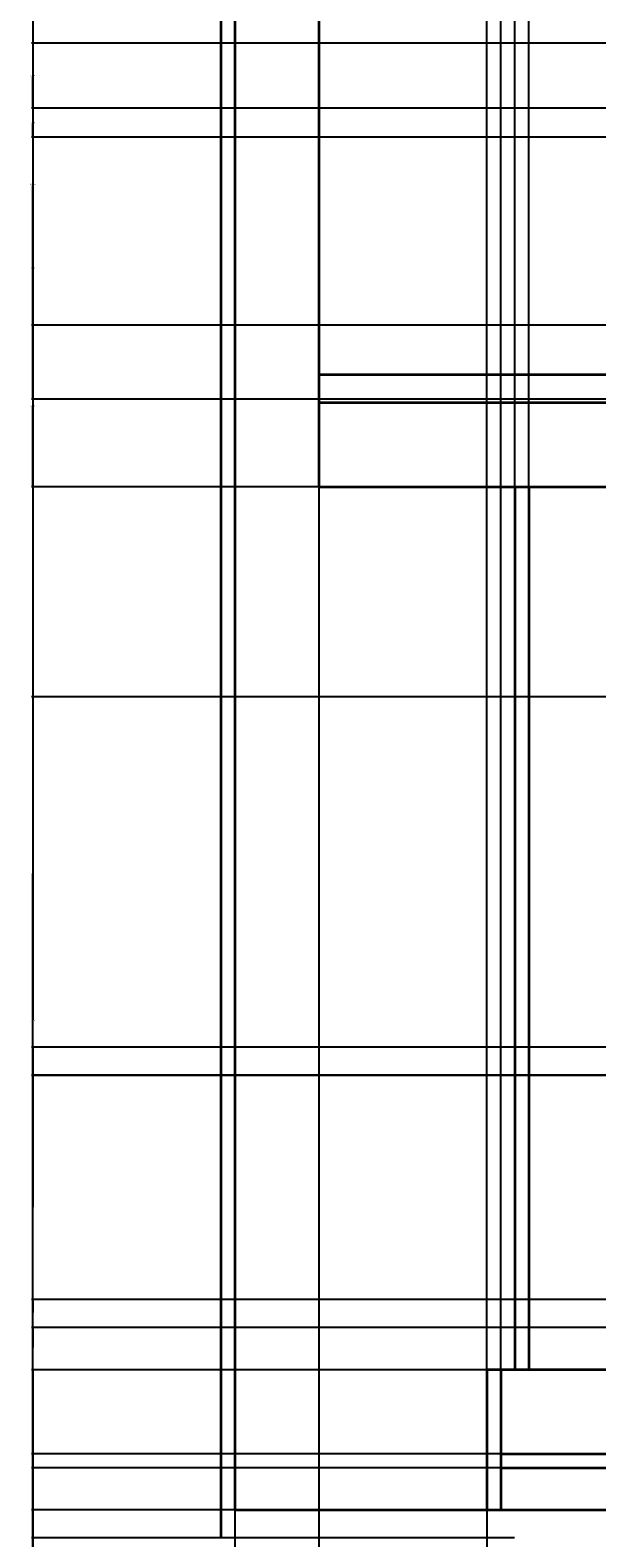
# Model space of a CAD drawing. Units: inches. Extents: x 2154 to 2740, y 571 to 1084.
# Tile 2 of 13: x 2154 to 2235, y 754 to 969. Entities that reach past the tile are written whole.
import ezdxf

# ---------------------------------------------------------------- set-up
doc = ezdxf.new("R2010")
doc.units = ezdxf.units.IN
for name, color, linetype, lineweight in [('A-ANNO-DIMS', 2, 'Continuous', 18), ('A-ELEV', 7, 'Continuous', 35), ('A-ROOF', 1, 'Continuous', 35)]:
    doc.layers.add(name, color=color, linetype=linetype, lineweight=lineweight)
doc.styles.get("Standard").update_dxf_attribs({"font": 'arial.ttf'})
doc.dimstyles.get("Standard").update_dxf_attribs({"dimtxt": 0.18, "dimasz": 0.18, "dimexe": 0.18, "dimexo": 0.0625, "dimgap": 0.09, "dimtad": 0, "dimtih": 1, "dimtoh": 1, "dimdec": 4, "dimzin": 0, "dimdsep": 46, "dimtxsty": 'Standard', "dimcen": 0.09, "dimadec": 0, "dimazin": 0, "dimtfac": 1, "dimtdec": 4, "dimtofl": 0, "dimtmove": 0, "dimatfit": 3, "dimfxl": 1, "dimtolj": 1, "dimtzin": 0, "dimarcsym": 0})

# ---------------------------------------------------------------- blocks, each defined once
blk = doc.blocks.new('*D10')
at = {"layer": 'A-ANNO-DIMS', "color": 0, "lineweight": -2, "transparency": 16777216}
for p, q in [((2447.14, 1057.01), (2154.18, 1057.01)), ((2154.36, 1056.83), (2154.36, 827.45)), ((2154.36, 597.71), (2154.36, 827.09)), ((2181.14, 597.53), (2154.18, 597.53))]:
    blk.add_line(p, q, dxfattribs=at)
at = {"layer": 'A-ANNO-DIMS', "color": 0, "transparency": 16777216}
for points in [[(2154.33, 1056.83), (2154.39, 1056.83), (2154.36, 1057.01)], [(2154.33, 597.71), (2154.39, 597.71), (2154.36, 597.53)]]:
    blk.add_solid(points, dxfattribs=at)
at = {"layer": 'Defpoints', "color": 0, "transparency": 16777216}
for p in [(2154.36, 1057.01), (2447.21, 1057.01), (2181.21, 597.53)]:
    blk.add_point(p, dxfattribs=at)
at = {"layer": 'A-ANNO-DIMS', "color": 0, "transparency": 16777216, "insert": (2154.36, 827.27), "char_height": 0.18, "attachment_point": 5}
blk.add_mtext('\\A1;459.5', dxfattribs=at)
blk = doc.blocks.new('*D14')
at = {"layer": 'A-ANNO-DIMS', "color": 0, "lineweight": -2, "transparency": 16777216}
for p, q in [((2221.14, 777.53), (2154.18, 777.53)), ((2154.36, 777.35), (2154.36, 687.71)), ((2154.36, 597.71), (2154.36, 687.35)), ((2223.14, 597.53), (2154.18, 597.53))]:
    blk.add_line(p, q, dxfattribs=at)
at = {"layer": 'A-ANNO-DIMS', "color": 0, "transparency": 16777216}
for points in [[(2154.33, 777.35), (2154.39, 777.35), (2154.36, 777.53)], [(2154.33, 597.71), (2154.39, 597.71), (2154.36, 597.53)]]:
    blk.add_solid(points, dxfattribs=at)
at = {"layer": 'Defpoints', "color": 0, "transparency": 16777216}
for p in [(2154.36, 777.53), (2221.21, 777.53), (2223.21, 597.53)]:
    blk.add_point(p, dxfattribs=at)
at = {"layer": 'A-ANNO-DIMS', "color": 0, "transparency": 16777216, "insert": (2154.36, 687.53), "char_height": 0.18, "attachment_point": 5}
blk.add_mtext('\\A1;180', dxfattribs=at)
blk = doc.blocks.new('*D15')
at = {"layer": 'A-ANNO-DIMS', "color": 0, "lineweight": -2, "transparency": 16777216}
for p, q in [((2223.14, 903.53), (2154.18, 903.53)), ((2154.36, 903.35), (2154.36, 840.71)), ((2154.36, 777.71), (2154.36, 840.35)), ((2221.14, 777.53), (2154.18, 777.53))]:
    blk.add_line(p, q, dxfattribs=at)
at = {"layer": 'A-ANNO-DIMS', "color": 0, "transparency": 16777216}
for points in [[(2154.33, 903.35), (2154.39, 903.35), (2154.36, 903.53)], [(2154.33, 777.71), (2154.39, 777.71), (2154.36, 777.53)]]:
    blk.add_solid(points, dxfattribs=at)
at = {"layer": 'Defpoints', "color": 0, "transparency": 16777216}
for p in [(2154.36, 903.53), (2223.21, 903.53), (2221.21, 777.53)]:
    blk.add_point(p, dxfattribs=at)
at = {"layer": 'A-ANNO-DIMS', "color": 0, "transparency": 16777216, "insert": (2154.36, 840.53), "char_height": 0.18, "attachment_point": 5}
blk.add_mtext('\\A1;126', dxfattribs=at)
blk = doc.blocks.new('*D30')
at = {"layer": 'A-ANNO-DIMS', "color": 0, "lineweight": -2, "transparency": 16777216}
for p, q in [((2657.14, 823.53), (2154.18, 823.53)), ((2154.36, 823.35), (2154.36, 800.71)), ((2154.36, 777.71), (2154.36, 800.35)), ((2657.14, 777.53), (2154.18, 777.53))]:
    blk.add_line(p, q, dxfattribs=at)
at = {"layer": 'A-ANNO-DIMS', "color": 0, "transparency": 16777216}
for points in [[(2154.33, 823.35), (2154.39, 823.35), (2154.36, 823.53)], [(2154.33, 777.71), (2154.39, 777.71), (2154.36, 777.53)]]:
    blk.add_solid(points, dxfattribs=at)
at = {"layer": 'Defpoints', "color": 0, "transparency": 16777216}
for p in [(2154.36, 823.53), (2657.21, 823.53), (2657.21, 777.53)]:
    blk.add_point(p, dxfattribs=at)
at = {"layer": 'A-ANNO-DIMS', "color": 0, "transparency": 16777216, "insert": (2154.36, 800.53), "char_height": 0.18, "attachment_point": 5}
blk.add_mtext('\\A1;46', dxfattribs=at)
blk = doc.blocks.new('*D33')
at = {"layer": 'A-ANNO-DIMS', "color": 0, "lineweight": -2, "transparency": 16777216}
for p, q in [((2412.64, 873.53), (2154.18, 873.53)), ((2154.36, 873.35), (2154.36, 848.71)), ((2154.36, 823.71), (2154.36, 848.35)), ((2412.64, 823.53), (2154.18, 823.53))]:
    blk.add_line(p, q, dxfattribs=at)
at = {"layer": 'A-ANNO-DIMS', "color": 0, "transparency": 16777216}
for points in [[(2154.33, 873.35), (2154.39, 873.35), (2154.36, 873.53)], [(2154.33, 823.71), (2154.39, 823.71), (2154.36, 823.53)]]:
    blk.add_solid(points, dxfattribs=at)
at = {"layer": 'Defpoints', "color": 0, "transparency": 16777216}
for p in [(2154.36, 873.53), (2412.71, 873.53), (2412.71, 823.53)]:
    blk.add_point(p, dxfattribs=at)
at = {"layer": 'A-ANNO-DIMS', "color": 0, "transparency": 16777216, "insert": (2154.36, 848.53), "char_height": 0.18, "attachment_point": 5}
blk.add_mtext('\\A1;50', dxfattribs=at)
blk = doc.blocks.new('*D35')
at = {"layer": 'A-ANNO-DIMS', "color": 0, "lineweight": -2, "transparency": 16777216}
for p, q in [((2447.21, 966.82), (2154.18, 966.82)), ((2154.36, 966.64), (2154.36, 946.87)), ((2154.36, 926.74), (2154.36, 946.51)), ((2284.14, 926.56), (2154.18, 926.56))]:
    blk.add_line(p, q, dxfattribs=at)
at = {"layer": 'A-ANNO-DIMS', "color": 0, "transparency": 16777216}
for points in [[(2154.33, 966.64), (2154.39, 966.64), (2154.36, 966.82)], [(2154.33, 926.74), (2154.39, 926.74), (2154.36, 926.56)]]:
    blk.add_solid(points, dxfattribs=at)
at = {"layer": 'Defpoints', "color": 0, "transparency": 16777216}
for p in [(2154.36, 966.82), (2447.27, 966.82), (2284.21, 926.56)]:
    blk.add_point(p, dxfattribs=at)
at = {"layer": 'A-ANNO-DIMS', "color": 0, "transparency": 16777216, "insert": (2154.36, 946.69), "char_height": 0.18, "attachment_point": 5}
blk.add_mtext('\\A1;40.255', dxfattribs=at)
blk = doc.blocks.new('*D36')
at = {"layer": 'A-ANNO-DIMS', "color": 0, "lineweight": -2, "transparency": 16777216}
for p, q in [((2447.21, 966.82), (2154.18, 966.82)), ((2154.36, 966.64), (2154.36, 962.36)), ((2154.36, 957.71), (2154.36, 961.99)), ((2447.14, 957.53), (2154.18, 957.53))]:
    blk.add_line(p, q, dxfattribs=at)
at = {"layer": 'A-ANNO-DIMS', "color": 0, "transparency": 16777216}
for points in [[(2154.33, 966.64), (2154.39, 966.64), (2154.36, 966.82)], [(2154.33, 957.71), (2154.39, 957.71), (2154.36, 957.53)]]:
    blk.add_solid(points, dxfattribs=at)
at = {"layer": 'Defpoints', "color": 0, "transparency": 16777216}
for p in [(2154.36, 966.82), (2447.27, 966.82), (2447.21, 957.53)]:
    blk.add_point(p, dxfattribs=at)
at = {"layer": 'A-ANNO-DIMS', "color": 0, "transparency": 16777216, "insert": (2154.36, 962.18), "char_height": 0.18, "attachment_point": 5}
blk.add_mtext('\\A1;9.287', dxfattribs=at)
blk = doc.blocks.new('*D37')
at = {"layer": 'A-ANNO-DIMS', "color": 0, "lineweight": -2, "transparency": 16777216}
for p, q in [((2447.14, 957.53), (2154.18, 957.53)), ((2154.36, 957.35), (2154.36, 955.65)), ((2154.36, 953.58), (2154.36, 955.29)), ((2447.11, 953.4), (2154.18, 953.4))]:
    blk.add_line(p, q, dxfattribs=at)
at = {"layer": 'A-ANNO-DIMS', "color": 0, "transparency": 16777216}
for points in [[(2154.33, 957.35), (2154.39, 957.35), (2154.36, 957.53)], [(2154.33, 953.58), (2154.39, 953.58), (2154.36, 953.4)]]:
    blk.add_solid(points, dxfattribs=at)
at = {"layer": 'Defpoints', "color": 0, "transparency": 16777216}
for p in [(2154.36, 957.53), (2447.21, 957.53), (2447.18, 953.4)]:
    blk.add_point(p, dxfattribs=at)
at = {"layer": 'A-ANNO-DIMS', "color": 0, "transparency": 16777216, "insert": (2154.36, 955.47), "char_height": 0.18, "attachment_point": 5}
blk.add_mtext('\\A1;4.127', dxfattribs=at)
blk = doc.blocks.new('*D38')
at = {"layer": 'A-ANNO-DIMS', "color": 0, "lineweight": -2, "transparency": 16777216}
for p, q in [((2447.11, 953.4), (2154.18, 953.4)), ((2154.36, 953.22), (2154.36, 934.9)), ((2154.36, 916.21), (2154.36, 934.53)), ((2295.71, 916.03), (2154.18, 916.03))]:
    blk.add_line(p, q, dxfattribs=at)
at = {"layer": 'A-ANNO-DIMS', "color": 0, "transparency": 16777216}
for points in [[(2154.33, 953.22), (2154.39, 953.22), (2154.36, 953.4)], [(2154.33, 916.21), (2154.39, 916.21), (2154.36, 916.03)]]:
    blk.add_solid(points, dxfattribs=at)
at = {"layer": 'Defpoints', "color": 0, "transparency": 16777216}
for p in [(2154.36, 953.4), (2447.18, 953.4), (2295.77, 916.03)]:
    blk.add_point(p, dxfattribs=at)
at = {"layer": 'A-ANNO-DIMS', "color": 0, "transparency": 16777216, "insert": (2154.36, 934.72), "char_height": 0.18, "attachment_point": 5}
blk.add_mtext('\\A1;37.38', dxfattribs=at)
blk = doc.blocks.new('*D39')
at = {"layer": 'A-ANNO-DIMS', "color": 0, "lineweight": -2, "transparency": 16777216}
for p, q in [((2183.21, 979.47), (2183.21, 570.5)), ((2417.21, 970.47), (2417.21, 570.5)), ((2183.39, 570.68), (2299.92, 570.68)), ((2417.03, 570.68), (2300.5, 570.68))]:
    blk.add_line(p, q, dxfattribs=at)
at = {"layer": 'A-ANNO-DIMS', "color": 0, "transparency": 16777216}
for points in [[(2183.39, 570.71), (2183.39, 570.65), (2183.21, 570.68)], [(2417.03, 570.71), (2417.03, 570.65), (2417.21, 570.68)]]:
    blk.add_solid(points, dxfattribs=at)
at = {"layer": 'Defpoints', "color": 0, "transparency": 16777216}
for p in [(2183.21, 979.53), (2417.21, 970.53), (2417.21, 570.68)]:
    blk.add_point(p, dxfattribs=at)
at = {"layer": 'A-ANNO-DIMS', "color": 0, "transparency": 16777216, "insert": (2300.21, 570.68), "char_height": 0.18, "attachment_point": 5}
blk.add_mtext('\\A1;234', dxfattribs=at)
blk = doc.blocks.new('*D46')
at = {"layer": 'A-ANNO-DIMS', "color": 0, "lineweight": -2, "transparency": 16777216}
for p, q in [((2195.27, 915.53), (2740.24, 915.53)), ((2740.06, 915.35), (2740.06, 909.71)), ((2740.06, 903.71), (2740.06, 909.35)), ((2195.27, 903.53), (2740.24, 903.53))]:
    blk.add_line(p, q, dxfattribs=at)
at = {"layer": 'A-ANNO-DIMS', "color": 0, "transparency": 16777216}
for points in [[(2740.03, 915.35), (2740.09, 915.35), (2740.06, 915.53)], [(2740.03, 903.71), (2740.09, 903.71), (2740.06, 903.53)]]:
    blk.add_solid(points, dxfattribs=at)
at = {"layer": 'Defpoints', "color": 0, "transparency": 16777216}
for p in [(2195.21, 915.53), (2740.06, 915.53), (2195.21, 903.53)]:
    blk.add_point(p, dxfattribs=at)
at = {"layer": 'A-ANNO-DIMS', "color": 0, "transparency": 16777216, "insert": (2740.06, 909.53), "char_height": 0.18, "attachment_point": 5}
blk.add_mtext('\\A1;12', dxfattribs=at)
blk = doc.blocks.new('*D47')
at = {"layer": 'A-ANNO-DIMS', "color": 0, "lineweight": -2, "transparency": 16777216}
for p, q in [((2195.269199, 919.532069), (2740.236699, 919.532069)), ((2740.056699, 919.352069), (2740.056699, 917.712069)), ((2740.056699, 915.712069), (2740.056699, 917.352069)), ((2195.269199, 915.532069), (2740.236699, 915.532069))]:
    blk.add_line(p, q, dxfattribs=at)
at = {"layer": 'A-ANNO-DIMS', "color": 0, "transparency": 16777216}
for points in [[(2740.026699, 919.352069), (2740.086699, 919.352069), (2740.056699, 919.532069)], [(2740.026699, 915.712069), (2740.086699, 915.712069), (2740.056699, 915.532069)]]:
    blk.add_solid(points, dxfattribs=at)
at = {"layer": 'Defpoints', "color": 0, "transparency": 16777216}
for p in [(2195.206699, 919.532069), (2740.056699, 919.532069), (2195.206699, 915.532069)]:
    blk.add_point(p, dxfattribs=at)
at = {"layer": 'A-ANNO-DIMS', "color": 0, "transparency": 16777216, "insert": (2740.056699, 917.532069), "char_height": 0.18, "attachment_point": 5}
blk.add_mtext('\\A1;4', dxfattribs=at)
blk = doc.blocks.new('*D48')
at = {"layer": 'A-ANNO-DIMS', "color": 0, "lineweight": -2, "transparency": 16777216}
for p, q in [((2195.27, 979.53), (2740.24, 979.53)), ((2740.06, 979.35), (2740.06, 949.71)), ((2740.06, 919.71), (2740.06, 949.35)), ((2195.27, 919.53), (2740.24, 919.53))]:
    blk.add_line(p, q, dxfattribs=at)
at = {"layer": 'A-ANNO-DIMS', "color": 0, "transparency": 16777216}
for points in [[(2740.03, 979.35), (2740.09, 979.35), (2740.06, 979.53)], [(2740.03, 919.71), (2740.09, 919.71), (2740.06, 919.53)]]:
    blk.add_solid(points, dxfattribs=at)
at = {"layer": 'Defpoints', "color": 0, "transparency": 16777216}
for p in [(2195.21, 979.53), (2740.06, 979.53), (2195.21, 919.53)]:
    blk.add_point(p, dxfattribs=at)
at = {"layer": 'A-ANNO-DIMS', "color": 0, "transparency": 16777216, "insert": (2740.06, 949.53), "char_height": 0.18, "attachment_point": 5}
blk.add_mtext('\\A1;60', dxfattribs=at)
blk = doc.blocks.new('*D51')
at = {"layer": 'A-ANNO-DIMS', "color": 0, "lineweight": -2, "transparency": 16777216}
for p, q in [((2183.21, 979.47), (2183.21, 570.5)), ((2195.21, 979.47), (2195.21, 570.5)), ((2183.39, 570.68), (2189, 570.68)), ((2195.03, 570.68), (2189.42, 570.68))]:
    blk.add_line(p, q, dxfattribs=at)
at = {"layer": 'A-ANNO-DIMS', "color": 0, "transparency": 16777216}
for points in [[(2183.39, 570.71), (2183.39, 570.65), (2183.21, 570.68)], [(2195.03, 570.71), (2195.03, 570.65), (2195.21, 570.68)]]:
    blk.add_solid(points, dxfattribs=at)
at = {"layer": 'Defpoints', "color": 0, "transparency": 16777216}
for p in [(2183.21, 979.53), (2195.21, 979.53), (2195.21, 570.68)]:
    blk.add_point(p, dxfattribs=at)
at = {"layer": 'A-ANNO-DIMS', "color": 0, "transparency": 16777216, "insert": (2189.21, 570.68), "char_height": 0.18, "attachment_point": 5}
blk.add_mtext('\\A1;12', dxfattribs=at)
blk = doc.blocks.new('*D54')
at = {"layer": 'A-ANNO-DIMS', "color": 0, "lineweight": -2, "transparency": 16777216}
for p, q in [((2284.14, 926.56), (2154.18, 926.56)), ((2154.36, 926.38), (2154.36, 915.23)), ((2154.36, 903.71), (2154.36, 914.87)), ((2284.14, 903.53), (2154.18, 903.53))]:
    blk.add_line(p, q, dxfattribs=at)
at = {"layer": 'A-ANNO-DIMS', "color": 0, "transparency": 16777216}
for points in [[(2154.33, 926.38), (2154.39, 926.38), (2154.36, 926.56)], [(2154.33, 903.71), (2154.39, 903.71), (2154.36, 903.53)]]:
    blk.add_solid(points, dxfattribs=at)
at = {"layer": 'Defpoints', "color": 0, "transparency": 16777216}
for p in [(2154.36, 926.56), (2284.21, 926.56), (2284.21, 903.53)]:
    blk.add_point(p, dxfattribs=at)
at = {"layer": 'A-ANNO-DIMS', "color": 0, "transparency": 16777216, "insert": (2154.36, 915.05), "char_height": 0.18, "attachment_point": 5}
blk.add_mtext('\\A1;23.03', dxfattribs=at)
blk = doc.blocks.new('*D57')
at = {"layer": 'A-ANNO-DIMS', "color": 0, "lineweight": -2, "transparency": 16777216}
for p, q in [((2219.144199, 757.532069), (2154.176699, 757.532069)), ((2154.356699, 757.352069), (2154.356699, 755.712069)), ((2154.356699, 753.712069), (2154.356699, 755.352069)), ((2223.144199, 753.532069), (2154.176699, 753.532069))]:
    blk.add_line(p, q, dxfattribs=at)
at = {"layer": 'A-ANNO-DIMS', "color": 0, "transparency": 16777216}
for points in [[(2154.326699, 757.352069), (2154.386699, 757.352069), (2154.356699, 757.532069)], [(2154.326699, 753.712069), (2154.386699, 753.712069), (2154.356699, 753.532069)]]:
    blk.add_solid(points, dxfattribs=at)
at = {"layer": 'Defpoints', "color": 0, "transparency": 16777216}
for p in [(2154.356699, 757.532069), (2219.206699, 757.532069), (2223.206699, 753.532069)]:
    blk.add_point(p, dxfattribs=at)
at = {"layer": 'A-ANNO-DIMS', "color": 0, "transparency": 16777216, "insert": (2154.356699, 755.532069), "char_height": 0.18, "attachment_point": 5}
blk.add_mtext('\\A1;4', dxfattribs=at)
blk = doc.blocks.new('*D58')
at = {"layer": 'A-ANNO-DIMS', "color": 0, "lineweight": -2, "transparency": 16777216}
for p, q in [((2221.14, 763.53), (2154.18, 763.53)), ((2154.36, 763.35), (2154.36, 760.71)), ((2154.36, 757.71), (2154.36, 760.35)), ((2219.14, 757.53), (2154.18, 757.53))]:
    blk.add_line(p, q, dxfattribs=at)
at = {"layer": 'A-ANNO-DIMS', "color": 0, "transparency": 16777216}
for points in [[(2154.33, 763.35), (2154.39, 763.35), (2154.36, 763.53)], [(2154.33, 757.71), (2154.39, 757.71), (2154.36, 757.53)]]:
    blk.add_solid(points, dxfattribs=at)
at = {"layer": 'Defpoints', "color": 0, "transparency": 16777216}
for p in [(2154.36, 763.53), (2221.21, 763.53), (2219.21, 757.53)]:
    blk.add_point(p, dxfattribs=at)
at = {"layer": 'A-ANNO-DIMS', "color": 0, "transparency": 16777216, "insert": (2154.36, 760.53), "char_height": 0.18, "attachment_point": 5}
blk.add_mtext('\\A1;6', dxfattribs=at)
blk = doc.blocks.new('*D59')
at = {"layer": 'A-ANNO-DIMS', "color": 0, "lineweight": -2, "transparency": 16777216}
for p, q in [((2221.14, 765.53), (2154.18, 765.53)), ((2154.36, 765.35), (2154.36, 764.71)), ((2154.36, 763.71), (2154.36, 764.35)), ((2221.14, 763.53), (2154.18, 763.53))]:
    blk.add_line(p, q, dxfattribs=at)
at = {"layer": 'A-ANNO-DIMS', "color": 0, "transparency": 16777216}
for points in [[(2154.33, 765.35), (2154.39, 765.35), (2154.36, 765.53)], [(2154.33, 763.71), (2154.39, 763.71), (2154.36, 763.53)]]:
    blk.add_solid(points, dxfattribs=at)
at = {"layer": 'Defpoints', "color": 0, "transparency": 16777216}
for p in [(2154.36, 765.53), (2221.21, 765.53), (2221.21, 763.53)]:
    blk.add_point(p, dxfattribs=at)
at = {"layer": 'A-ANNO-DIMS', "color": 0, "transparency": 16777216, "insert": (2154.36, 764.53), "char_height": 0.18, "attachment_point": 5}
blk.add_mtext('\\A1;2', dxfattribs=at)
blk = doc.blocks.new('*D60')
at = {"layer": 'A-ANNO-DIMS', "color": 0, "lineweight": -2, "transparency": 16777216}
for p, q in [((2219.14, 777.53), (2154.18, 777.53)), ((2154.36, 777.35), (2154.36, 771.71)), ((2154.36, 765.71), (2154.36, 771.35)), ((2221.14, 765.53), (2154.18, 765.53))]:
    blk.add_line(p, q, dxfattribs=at)
at = {"layer": 'A-ANNO-DIMS', "color": 0, "transparency": 16777216}
for points in [[(2154.33, 777.35), (2154.39, 777.35), (2154.36, 777.53)], [(2154.33, 765.71), (2154.39, 765.71), (2154.36, 765.53)]]:
    blk.add_solid(points, dxfattribs=at)
at = {"layer": 'Defpoints', "color": 0, "transparency": 16777216}
for p in [(2154.36, 777.53), (2219.21, 777.53), (2221.21, 765.53)]:
    blk.add_point(p, dxfattribs=at)
at = {"layer": 'A-ANNO-DIMS', "color": 0, "transparency": 16777216, "insert": (2154.36, 771.53), "char_height": 0.18, "attachment_point": 5}
blk.add_mtext('\\A1;12', dxfattribs=at)
blk = doc.blocks.new('*D61')
at = {"layer": 'A-ANNO-DIMS', "color": 0, "lineweight": -2, "transparency": 16777216}
for p, q in [((2183.21, 757.47), (2183.21, 570.5)), ((2219.21, 757.47), (2219.21, 570.5)), ((2183.39, 570.68), (2200.99, 570.68)), ((2219.03, 570.68), (2201.43, 570.68))]:
    blk.add_line(p, q, dxfattribs=at)
at = {"layer": 'A-ANNO-DIMS', "color": 0, "transparency": 16777216}
for points in [[(2183.39, 570.71), (2183.39, 570.65), (2183.21, 570.68)], [(2219.03, 570.71), (2219.03, 570.65), (2219.21, 570.68)]]:
    blk.add_solid(points, dxfattribs=at)
at = {"layer": 'Defpoints', "color": 0, "transparency": 16777216}
for p in [(2183.21, 757.53), (2219.21, 757.53), (2219.21, 570.68)]:
    blk.add_point(p, dxfattribs=at)
at = {"layer": 'A-ANNO-DIMS', "color": 0, "transparency": 16777216, "insert": (2201.21, 570.68), "char_height": 0.18, "attachment_point": 5}
blk.add_mtext('\\A1;36', dxfattribs=at)
blk = doc.blocks.new('*D62')
at = {"layer": 'A-ANNO-DIMS', "color": 0, "lineweight": -2, "transparency": 16777216}
for p, q in [((2219.21, 777.59), (2219.21, 1084.04)), ((2219.39, 1083.86), (2220.06, 1083.86)), ((2221.03, 1083.86), (2220.36, 1083.86)), ((2221.21, 777.59), (2221.21, 1084.04))]:
    blk.add_line(p, q, dxfattribs=at)
at = {"layer": 'A-ANNO-DIMS', "color": 0, "transparency": 16777216}
for points in [[(2219.39, 1083.89), (2219.39, 1083.83), (2219.21, 1083.86)], [(2221.03, 1083.89), (2221.03, 1083.83), (2221.21, 1083.86)]]:
    blk.add_solid(points, dxfattribs=at)
at = {"layer": 'Defpoints', "color": 0, "transparency": 16777216}
for p in [(2221.21, 1083.86), (2219.21, 777.53), (2221.21, 777.53)]:
    blk.add_point(p, dxfattribs=at)
at = {"layer": 'A-ANNO-DIMS', "color": 0, "transparency": 16777216, "insert": (2220.21, 1083.86), "char_height": 0.18, "attachment_point": 5}
blk.add_mtext('\\A1;2', dxfattribs=at)
blk = doc.blocks.new('*D63')
at = {"layer": 'A-ANNO-DIMS', "color": 0, "lineweight": -2, "transparency": 16777216}
for p, q in [((2221.21, 777.59), (2221.21, 1084.04)), ((2221.39, 1083.86), (2222.06, 1083.86)), ((2223.03, 1083.86), (2222.36, 1083.86)), ((2223.21, 777.59), (2223.21, 1084.04))]:
    blk.add_line(p, q, dxfattribs=at)
at = {"layer": 'A-ANNO-DIMS', "color": 0, "transparency": 16777216}
for points in [[(2221.39, 1083.89), (2221.39, 1083.83), (2221.21, 1083.86)], [(2223.03, 1083.89), (2223.03, 1083.83), (2223.21, 1083.86)]]:
    blk.add_solid(points, dxfattribs=at)
at = {"layer": 'Defpoints', "color": 0, "transparency": 16777216}
for p in [(2223.21, 1083.86), (2221.21, 777.53), (2223.21, 777.53)]:
    blk.add_point(p, dxfattribs=at)
at = {"layer": 'A-ANNO-DIMS', "color": 0, "transparency": 16777216, "insert": (2222.21, 1083.86), "char_height": 0.18, "attachment_point": 5}
blk.add_mtext('\\A1;2', dxfattribs=at)
blk = doc.blocks.new('*D64')
at = {"layer": 'A-ANNO-DIMS', "color": 0, "lineweight": -2, "transparency": 16777216}
for p, q in [((2223.21, 777.59), (2223.21, 1084.04)), ((2223.39, 1083.86), (2224.06, 1083.86)), ((2225.03, 1083.86), (2224.36, 1083.86)), ((2225.21, 777.59), (2225.21, 1084.04))]:
    blk.add_line(p, q, dxfattribs=at)
at = {"layer": 'A-ANNO-DIMS', "color": 0, "transparency": 16777216}
for points in [[(2223.39, 1083.89), (2223.39, 1083.83), (2223.21, 1083.86)], [(2225.03, 1083.89), (2225.03, 1083.83), (2225.21, 1083.86)]]:
    blk.add_solid(points, dxfattribs=at)
at = {"layer": 'Defpoints', "color": 0, "transparency": 16777216}
for p in [(2225.21, 1083.86), (2223.21, 777.53), (2225.21, 777.53)]:
    blk.add_point(p, dxfattribs=at)
at = {"layer": 'A-ANNO-DIMS', "color": 0, "transparency": 16777216, "insert": (2224.21, 1083.86), "char_height": 0.18, "attachment_point": 5}
blk.add_mtext('\\A1;2', dxfattribs=at)
blk = doc.blocks.new('*D65')
at = {"layer": 'A-ANNO-DIMS', "color": 0, "lineweight": -2, "transparency": 16777216}
for p, q in [((2225.21, 777.59), (2225.21, 1084.04)), ((2225.39, 1083.86), (2231, 1083.86)), ((2237.03, 1083.86), (2231.42, 1083.86)), ((2237.21, 777.59), (2237.21, 1084.04))]:
    blk.add_line(p, q, dxfattribs=at)
at = {"layer": 'A-ANNO-DIMS', "color": 0, "transparency": 16777216}
for points in [[(2225.39, 1083.89), (2225.39, 1083.83), (2225.21, 1083.86)], [(2237.03, 1083.89), (2237.03, 1083.83), (2237.21, 1083.86)]]:
    blk.add_solid(points, dxfattribs=at)
at = {"layer": 'Defpoints', "color": 0, "transparency": 16777216}
for p in [(2237.21, 1083.86), (2225.21, 777.53), (2237.21, 777.53)]:
    blk.add_point(p, dxfattribs=at)
at = {"layer": 'A-ANNO-DIMS', "color": 0, "transparency": 16777216, "insert": (2231.21, 1083.86), "char_height": 0.18, "attachment_point": 5}
blk.add_mtext('\\A1;12', dxfattribs=at)
blk = doc.blocks.new('*D122')
at = {"layer": 'A-ANNO-DIMS', "color": 0, "lineweight": -2, "transparency": 16777216}
for p, q in [((2237.14, 783.53), (2154.18, 783.53)), ((2154.36, 783.35), (2154.36, 780.71)), ((2154.36, 777.71), (2154.36, 780.35)), ((2237.14, 777.53), (2154.18, 777.53))]:
    blk.add_line(p, q, dxfattribs=at)
at = {"layer": 'A-ANNO-DIMS', "color": 0, "transparency": 16777216}
for points in [[(2154.33, 783.35), (2154.39, 783.35), (2154.36, 783.53)], [(2154.33, 777.71), (2154.39, 777.71), (2154.36, 777.53)]]:
    blk.add_solid(points, dxfattribs=at)
at = {"layer": 'Defpoints', "color": 0, "transparency": 16777216}
for p in [(2154.36, 783.53), (2237.21, 783.53), (2237.21, 777.53)]:
    blk.add_point(p, dxfattribs=at)
at = {"layer": 'A-ANNO-DIMS', "color": 0, "transparency": 16777216, "insert": (2154.36, 780.53), "char_height": 0.18, "attachment_point": 5}
blk.add_mtext('\\A1;6', dxfattribs=at)
blk = doc.blocks.new('*D123')
at = {"layer": 'A-ANNO-DIMS', "color": 0, "lineweight": -2, "transparency": 16777216}
for p, q in [((2237.144199, 787.532069), (2154.176699, 787.532069)), ((2154.356699, 787.352069), (2154.356699, 785.712069)), ((2154.356699, 783.712069), (2154.356699, 785.352069)), ((2237.144199, 783.532069), (2154.176699, 783.532069))]:
    blk.add_line(p, q, dxfattribs=at)
at = {"layer": 'A-ANNO-DIMS', "color": 0, "transparency": 16777216}
for points in [[(2154.326699, 787.352069), (2154.386699, 787.352069), (2154.356699, 787.532069)], [(2154.326699, 783.712069), (2154.386699, 783.712069), (2154.356699, 783.532069)]]:
    blk.add_solid(points, dxfattribs=at)
at = {"layer": 'Defpoints', "color": 0, "transparency": 16777216}
for p in [(2154.356699, 787.532069), (2237.206699, 787.532069), (2237.206699, 783.532069)]:
    blk.add_point(p, dxfattribs=at)
at = {"layer": 'A-ANNO-DIMS', "color": 0, "transparency": 16777216, "insert": (2154.356699, 785.532069), "char_height": 0.18, "attachment_point": 5}
blk.add_mtext('\\A1;4', dxfattribs=at)
blk = doc.blocks.new('*D124')
at = {"layer": 'A-ANNO-DIMS', "color": 0, "lineweight": -2, "transparency": 16777216}
for p, q in [((2237.14, 819.53), (2154.18, 819.53)), ((2154.36, 819.35), (2154.36, 803.71)), ((2154.36, 787.71), (2154.36, 803.35)), ((2237.14, 787.53), (2154.18, 787.53))]:
    blk.add_line(p, q, dxfattribs=at)
at = {"layer": 'A-ANNO-DIMS', "color": 0, "transparency": 16777216}
for points in [[(2154.33, 819.35), (2154.39, 819.35), (2154.36, 819.53)], [(2154.33, 787.71), (2154.39, 787.71), (2154.36, 787.53)]]:
    blk.add_solid(points, dxfattribs=at)
at = {"layer": 'Defpoints', "color": 0, "transparency": 16777216}
for p in [(2154.36, 819.53), (2237.21, 819.53), (2237.21, 787.53)]:
    blk.add_point(p, dxfattribs=at)
at = {"layer": 'A-ANNO-DIMS', "color": 0, "transparency": 16777216, "insert": (2154.36, 803.53), "char_height": 0.18, "attachment_point": 5}
blk.add_mtext('\\A1;32', dxfattribs=at)
blk = doc.blocks.new('*D125')
at = {"layer": 'A-ANNO-DIMS', "color": 0, "lineweight": -2, "transparency": 16777216}
for p, q in [((2237.144199, 823.532069), (2154.176699, 823.532069)), ((2154.356699, 823.352069), (2154.356699, 821.712069)), ((2154.356699, 819.712069), (2154.356699, 821.352069)), ((2237.144199, 819.532069), (2154.176699, 819.532069))]:
    blk.add_line(p, q, dxfattribs=at)
at = {"layer": 'A-ANNO-DIMS', "color": 0, "transparency": 16777216}
for points in [[(2154.326699, 823.352069), (2154.386699, 823.352069), (2154.356699, 823.532069)], [(2154.326699, 819.712069), (2154.386699, 819.712069), (2154.356699, 819.532069)]]:
    blk.add_solid(points, dxfattribs=at)
at = {"layer": 'Defpoints', "color": 0, "transparency": 16777216}
for p in [(2154.356699, 823.532069), (2237.206699, 823.532069), (2237.206699, 819.532069)]:
    blk.add_point(p, dxfattribs=at)
at = {"layer": 'A-ANNO-DIMS', "color": 0, "transparency": 16777216, "insert": (2154.356699, 821.532069), "char_height": 0.18, "attachment_point": 5}
blk.add_mtext('\\A1;4', dxfattribs=at)

msp = doc.modelspace()

# ---------------------------------------------------------------- linework, layer by layer
at = {"layer": 'A-ELEV'}
for p, q in [((2181.2067, 981.5321), (2181.2067, 753.5321)), ((2183.2067, 979.5321), (2183.2067, 757.5321)), ((2223.2067, 903.5321), (2223.2067, 777.5321)), ((2225.2067, 903.5321), (2225.2067, 777.5321)), ((2219.2067, 777.5321), (2219.2067, 757.5321)), ((2219.2067, 777.5321), (2675.2067, 777.5321)), ((2221.2067, 777.5321), (2221.2067, 757.5321)), ((2221.2067, 765.5321), (2673.2067, 765.5321)), ((2221.2067, 763.5321), (2673.2067, 763.5321)), ((2183.2067, 757.5321), (2711.2067, 757.5321))]:
    msp.add_line(p, q, dxfattribs=at)
at = {"layer": 'A-ROOF'}
for p, q in [((2195.2067, 979.5321), (2195.2067, 903.5321)), ((2195.2067, 919.5321), (2295.7729, 919.5321)), ((2195.2067, 915.5321), (2699.2067, 915.5321)), ((2195.2067, 903.5321), (2699.2067, 903.5321))]:
    msp.add_line(p, q, dxfattribs=at)

# ---------------------------------------------------------------- dimensions: what is measured, and where the dimension line sits
at = {"layer": 'A-ANNO-DIMS'}
for base, p1, p2, picture, middle in [((2221.2067, 1083.8553), (2219.2067, 777.5321), (2221.2067, 777.5321), '*D62', (2220.2067, 1083.8553)), ((2223.2067, 1083.8553), (2221.2067, 777.5321), (2223.2067, 777.5321), '*D63', (2222.2067, 1083.8553)), ((2225.2067, 1083.8553), (2223.2067, 777.5321), (2225.2067, 777.5321), '*D64', (2224.2067, 1083.8553)), ((2237.2067, 1083.8553), (2225.2067, 777.5321), (2237.2067, 777.5321), '*D65', (2231.2067, 1083.8553)), ((2417.2067, 570.6821), (2183.2067, 979.5321), (2417.2067, 970.5321), '*D39', (2300.2067, 570.6821)), ((2195.2067, 570.6821), (2183.2067, 979.5321), (2195.2067, 979.5321), '*D51', (2189.2067, 570.6821)), ((2219.2067, 570.6821), (2183.2067, 757.5321), (2219.2067, 757.5321), '*D61', (2201.2067, 570.6821))]:
    dim = msp.add_linear_dim(base=base, p1=p1, p2=p2, dimstyle='Standard', override={"dimdec": 0, "dimlfac": 1, "dimrnd": 0, "dimzin": 0, "dimdsep": 46, "dimlunit": 2}, dxfattribs=at)
    dim.commit()
    dim.dimension.update_dxf_attribs({"geometry": picture, "text_midpoint": middle})
for base, p1, p2, override, picture, middle in [((2154.3567, 1057.0053), (2181.2067, 597.5321), (2447.2067, 1057.0053), {"dimdec": 1, "dimlfac": 1, "dimrnd": 0, "dimzin": 0, "dimdsep": 46, "dimlunit": 2}, '*D10', (2154.3567, 827.2687)), ((2740.0567, 979.5321), (2195.2067, 919.5321), (2195.2067, 979.5321), {"dimdec": 0, "dimlfac": 1, "dimrnd": 0, "dimzin": 0, "dimdsep": 46, "dimlunit": 2}, '*D48', (2740.0567, 949.5321)), ((2154.3567, 966.8186), (2284.2067, 926.5633), (2447.273, 966.8186), {"dimdec": 3, "dimlfac": 1, "dimrnd": 0, "dimzin": 0, "dimdsep": 46, "dimlunit": 2}, '*D35', (2154.3567, 946.691)), ((2154.3567, 966.81862), (2447.2067, 957.53207), (2447.273, 966.81862), {"dimdec": 3, "dimlfac": 1, "dimrnd": 0, "dimzin": 0, "dimdsep": 46, "dimlunit": 2}, '*D36', (2154.3567, 962.17534)), ((2154.3567, 957.5321), (2447.1772, 953.4047), (2447.2067, 957.5321), {"dimdec": 3, "dimlfac": 1, "dimrnd": 0, "dimzin": 0, "dimdsep": 46, "dimlunit": 2}, '*D37', (2154.3567, 955.4684)), ((2154.3567, 953.4047), (2295.7714, 916.028), (2447.1772, 953.4047), {"dimdec": 2, "dimlfac": 1, "dimrnd": 0, "dimzin": 0, "dimdsep": 46, "dimlunit": 2}, '*D38', (2154.3567, 934.7163)), ((2154.3567, 926.5633), (2284.2067, 903.5321), (2284.2067, 926.5633), {"dimdec": 2, "dimlfac": 1, "dimrnd": 0, "dimzin": 0, "dimdsep": 46, "dimlunit": 2}, '*D54', (2154.3567, 915.0477)), ((2740.0567, 919.5321), (2195.2067, 915.5321), (2195.2067, 919.5321), {"dimdec": 0, "dimlfac": 1, "dimrnd": 0, "dimzin": 0, "dimdsep": 46, "dimlunit": 2}, '*D47', (2740.0567, 917.5321)), ((2740.0567, 915.5321), (2195.2067, 903.5321), (2195.2067, 915.5321), {"dimdec": 0, "dimlfac": 1, "dimrnd": 0, "dimzin": 0, "dimdsep": 46, "dimlunit": 2}, '*D46', (2740.0567, 909.5321)), ((2154.3567, 903.5321), (2221.2067, 777.5321), (2223.2067, 903.5321), {"dimdec": 0, "dimlfac": 1, "dimrnd": 0, "dimzin": 0, "dimdsep": 46, "dimlunit": 2}, '*D15', (2154.3567, 840.5321)), ((2154.3567, 873.5321), (2412.7067, 823.5321), (2412.7067, 873.5321), {"dimdec": 0, "dimlfac": 1, "dimrnd": 0, "dimzin": 0, "dimdsep": 46, "dimlunit": 2}, '*D33', (2154.3567, 848.5321)), ((2154.3567, 823.5321), (2657.2067, 777.5321), (2657.2067, 823.5321), {"dimdec": 0, "dimlfac": 1, "dimrnd": 0, "dimzin": 0, "dimdsep": 46, "dimlunit": 2}, '*D30', (2154.3567, 800.5321)), ((2154.3567, 823.5321), (2237.2067, 819.5321), (2237.2067, 823.5321), {"dimdec": 0, "dimlfac": 1, "dimrnd": 0, "dimzin": 0, "dimdsep": 46, "dimlunit": 2}, '*D125', (2154.3567, 821.5321)), ((2154.3567, 819.5321), (2237.2067, 787.5321), (2237.2067, 819.5321), {"dimdec": 0, "dimlfac": 1, "dimrnd": 0, "dimzin": 0, "dimdsep": 46, "dimlunit": 2}, '*D124', (2154.3567, 803.5321)), ((2154.3567, 787.5321), (2237.2067, 783.5321), (2237.2067, 787.5321), {"dimdec": 0, "dimlfac": 1, "dimrnd": 0, "dimzin": 0, "dimdsep": 46, "dimlunit": 2}, '*D123', (2154.3567, 785.5321)), ((2154.3567, 783.5321), (2237.2067, 777.5321), (2237.2067, 783.5321), {"dimdec": 0, "dimlfac": 1, "dimrnd": 0, "dimzin": 0, "dimdsep": 46, "dimlunit": 2}, '*D122', (2154.3567, 780.5321)), ((2154.3567, 777.5321), (2223.2067, 597.5321), (2221.2067, 777.5321), {"dimdec": 0, "dimlfac": 1, "dimrnd": 0, "dimzin": 0, "dimdsep": 46, "dimlunit": 2}, '*D14', (2154.3567, 687.5321)), ((2154.3567, 777.5321), (2221.2067, 765.5321), (2219.2067, 777.5321), {"dimdec": 0, "dimlfac": 1, "dimrnd": 0, "dimzin": 0, "dimdsep": 46, "dimlunit": 2}, '*D60', (2154.3567, 771.5321)), ((2154.3567, 765.5321), (2221.2067, 763.5321), (2221.2067, 765.5321), {"dimdec": 0, "dimlfac": 1, "dimrnd": 0, "dimzin": 0, "dimdsep": 46, "dimlunit": 2}, '*D59', (2154.3567, 764.5321)), ((2154.3567, 763.5321), (2219.2067, 757.5321), (2221.2067, 763.5321), {"dimdec": 0, "dimlfac": 1, "dimrnd": 0, "dimzin": 0, "dimdsep": 46, "dimlunit": 2}, '*D58', (2154.3567, 760.5321)), ((2154.3567, 757.5321), (2223.2067, 753.5321), (2219.2067, 757.5321), {"dimdec": 0, "dimlfac": 1, "dimrnd": 0, "dimzin": 0, "dimdsep": 46, "dimlunit": 2}, '*D57', (2154.3567, 755.5321))]:
    dim = msp.add_linear_dim(base=base, p1=p1, p2=p2, angle=90, dimstyle='Standard', override=override, dxfattribs=at)
    dim.commit()
    dim.dimension.update_dxf_attribs({"geometry": picture, "text_midpoint": middle})

doc.saveas('drawing.dxf')
